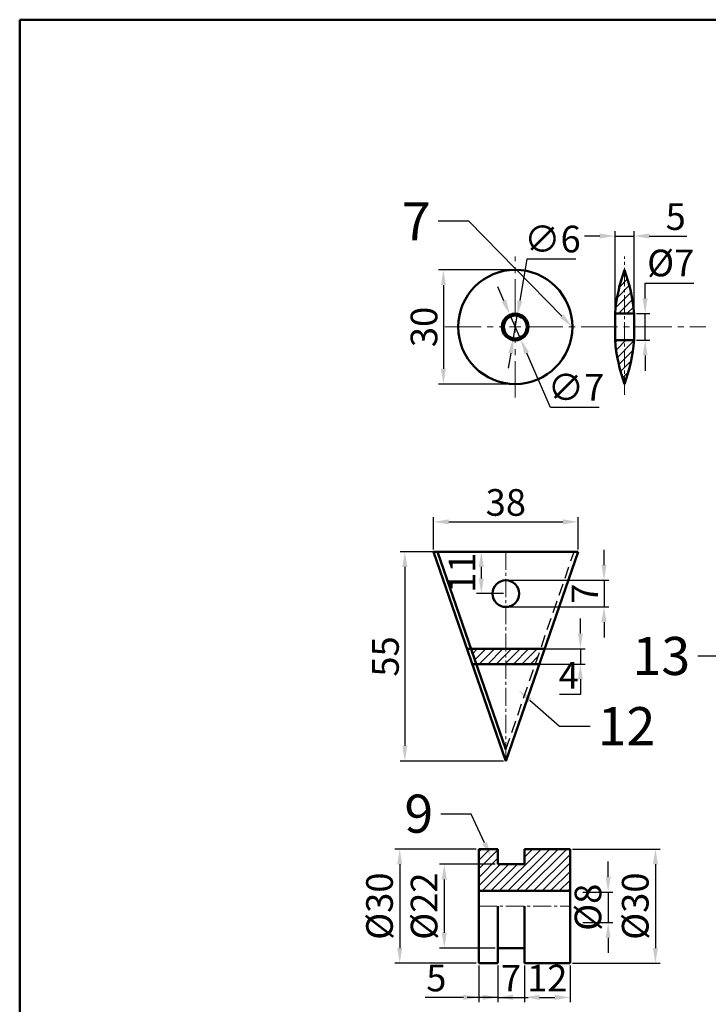
# Model space of a CAD drawing. Units: millimetres. Extents: x 376 to 1043, y -28 to 427.
# Tile 2 of 5: x 376 to 557, y 168 to 427. Entities that reach past the tile are written whole.
import ezdxf
from ezdxf import colors
from ezdxf.entities.mleader import LeaderData, LeaderLine
from ezdxf.math import Vec2, Vec3

# ---------------------------------------------------------------- set-up
doc = ezdxf.new("R2010")
doc.units = ezdxf.units.MM
doc.header["$LTSCALE"] = 0.5
doc.linetypes.add('CENTER2', pattern=[28.575, 19.05, -3.175, 3.175, -3.175])
doc.linetypes.add('DASHED', pattern=[19.05, 12.7, -6.35])
for name, color, linetype, lineweight in [('M-CNTR', 1, 'CENTER2', 18), ('M-DIMS', 2, 'Continuous', 25), ('M-HATC', 8, 'Continuous', 18), ('M-HIDN', 4, 'DASHED', 25), ('M-OUTL', 7, 'Continuous', 50)]:
    doc.layers.add(name, color=color, linetype=linetype, lineweight=lineweight)
doc.styles.get("Standard").update_dxf_attribs({"font": 'arial.ttf'})
doc.dimstyles.new('ISO-25', dxfattribs={"dimtxt": 7, "dimasz": 4, "dimexe": 1.25, "dimexo": 0.625, "dimtad": 1, "dimtoh": 1, "dimtxsty": 'Standard', "dimcen": 2.5, "dimadec": 0, "dimazin": 0, "dimtfac": 1, "dimtmove": 0, "dimatfit": 3, "dimfxl": 1, "dimarcsym": 0})

# ---------------------------------------------------------------- blocks, each defined once
blk = doc.blocks.new('*U36')
at = {"layer": 'M-CNTR', "color": 0, "transparency": 16777216}
for p, q in [((0, 3), (0, 18.5)), ((-18.5, 0), (-3, 0)), ((3, 0), (50.08, 0)), ((0, -18.5), (0, -3))]:
    blk.add_line(p, q, dxfattribs=at)
at = {"layer": 'M-CNTR', "color": 0, "linetype": 'Continuous', "transparency": 16777216}
for p, q in [((-1.5, 0), (1.5, 0)), ((0, -1.5), (0, 1.5))]:
    blk.add_line(p, q, dxfattribs=at)
blk = doc.blocks.new('*D37')
at = {"layer": 'Defpoints', "color": 0, "ltscale": 0.5, "transparency": 16777216}
for p in [(537.84, 370.17), (532.84, 346.29), (537.84, 346.29)]:
    blk.add_point(p, dxfattribs=at)
at = {"layer": 'M-DIMS', "color": 0, "lineweight": -2, "ltscale": 0.5, "transparency": 16777216}
for p, q in [((528.84, 370.17), (524.84, 370.17)), ((532.84, 346.91), (532.84, 371.42)), ((532.84, 370.17), (537.84, 370.17)), ((537.84, 346.91), (537.84, 371.42)), ((541.84, 370.17), (551.73, 370.17))]:
    blk.add_line(p, q, dxfattribs=at)
at = {"layer": 'M-DIMS', "color": 0, "ltscale": 0.5, "transparency": 16777216}
for points in [[(528.84, 370.84), (528.84, 369.5), (532.84, 370.17)], [(541.84, 370.84), (541.84, 369.5), (537.84, 370.17)]]:
    blk.add_solid(points, dxfattribs=at)
at = {"layer": 'M-DIMS', "color": 0, "ltscale": 0.5, "transparency": 16777216, "insert": (548.78, 374.36), "char_height": 7, "attachment_point": 5}
blk.add_mtext('5', dxfattribs=at)
blk = doc.blocks.new('*D38')
at = {"layer": 'Defpoints', "color": 0, "ltscale": 0.5, "transparency": 16777216}
for p in [(537.84, 349.79), (537.84, 342.79), (540.75, 342.79)]:
    blk.add_point(p, dxfattribs=at)
at = {"layer": 'M-DIMS', "color": 0, "lineweight": -2, "ltscale": 0.5, "transparency": 16777216}
for p, q in [((540.75, 353.79), (540.75, 357.79)), ((540.75, 357.79), (553.58, 357.79)), ((538.46, 349.79), (542, 349.79)), ((540.75, 342.79), (540.75, 349.79)), ((538.46, 342.79), (542, 342.79)), ((540.75, 338.79), (540.75, 334.79))]:
    blk.add_line(p, q, dxfattribs=at)
at = {"layer": 'M-DIMS', "color": 0, "ltscale": 0.5, "transparency": 16777216}
for points in [[(540.08, 353.79), (541.41, 353.79), (540.75, 349.79)], [(540.08, 338.79), (541.41, 338.79), (540.75, 342.79)]]:
    blk.add_solid(points, dxfattribs=at)
at = {"layer": 'M-DIMS', "color": 0, "ltscale": 0.5, "transparency": 16777216, "insert": (547.47, 362.18), "char_height": 7, "attachment_point": 5}
blk.add_mtext('%%C7', dxfattribs=at)
blk = doc.blocks.new('*D39')
at = {"layer": 'Defpoints', "color": 0, "ltscale": 0.5, "transparency": 16777216}
for p in [(506.64, 361.29), (487.76, 331.29), (506.64, 331.29)]:
    blk.add_point(p, dxfattribs=at)
at = {"layer": 'M-DIMS', "color": 0, "lineweight": -2, "ltscale": 0.5, "transparency": 16777216}
for p, q in [((506.01, 361.29), (486.51, 361.29)), ((487.76, 357.29), (487.76, 335.29)), ((506.01, 331.29), (486.51, 331.29))]:
    blk.add_line(p, q, dxfattribs=at)
at = {"layer": 'M-DIMS', "color": 0, "ltscale": 0.5, "transparency": 16777216}
for points in [[(487.09, 357.29), (488.42, 357.29), (487.76, 361.29)], [(487.09, 335.29), (488.42, 335.29), (487.76, 331.29)]]:
    blk.add_solid(points, dxfattribs=at)
at = {"layer": 'M-DIMS', "color": 0, "ltscale": 0.5, "transparency": 16777216, "insert": (483.56, 346.29), "char_height": 7, "attachment_point": 5, "rotation": 90}
blk.add_mtext('30', dxfattribs=at)
blk = doc.blocks.new('*D40')
at = {"layer": 'Defpoints', "color": 0, "ltscale": 0.5, "transparency": 16777216}
for p in [(505.24, 349.5), (508.04, 343.08)]:
    blk.add_point(p, dxfattribs=at)
at = {"layer": 'M-DIMS', "color": 0, "lineweight": -2, "ltscale": 0.5, "transparency": 16777216}
for p, q in [((503.64, 353.16), (502.04, 356.83)), ((505.24, 349.5), (508.04, 343.08)), ((515.86, 325.14), (509.64, 339.41)), ((528.69, 325.14), (515.86, 325.14))]:
    blk.add_line(p, q, dxfattribs=at)
at = {"layer": 'M-DIMS', "color": 0, "ltscale": 0.5, "transparency": 16777216}
for points in [[(504.25, 353.43), (503.03, 352.9), (505.24, 349.5)], [(510.25, 339.68), (509.03, 339.15), (508.04, 343.08)]]:
    blk.add_solid(points, dxfattribs=at)
at = {"layer": 'M-DIMS', "color": 0, "ltscale": 0.5, "transparency": 16777216, "insert": (522.59, 329.53), "char_height": 7, "attachment_point": 5}
blk.add_mtext('∅7', dxfattribs=at)
blk = doc.blocks.new('*D41')
at = {"layer": 'Defpoints', "color": 0, "ltscale": 0.5, "transparency": 16777216}
for p in [(507.15, 349.24), (506.13, 343.33)]:
    blk.add_point(p, dxfattribs=at)
at = {"layer": 'M-DIMS', "color": 0, "lineweight": -2, "ltscale": 0.5, "transparency": 16777216}
for p, q in [((509.68, 364.07), (507.82, 353.19)), ((522.51, 364.07), (509.68, 364.07)), ((506.13, 343.33), (507.15, 349.24)), ((505.46, 339.39), (504.78, 335.44))]:
    blk.add_line(p, q, dxfattribs=at)
at = {"layer": 'M-DIMS', "color": 0, "ltscale": 0.5, "transparency": 16777216}
for points in [[(507.16, 353.3), (508.48, 353.07), (507.15, 349.24)], [(504.8, 339.5), (506.12, 339.27), (506.13, 343.33)]]:
    blk.add_solid(points, dxfattribs=at)
at = {"layer": 'M-DIMS', "color": 0, "ltscale": 0.5, "transparency": 16777216, "insert": (516.41, 368.47), "char_height": 7, "attachment_point": 5}
blk.add_mtext('∅6', dxfattribs=at)
blk = doc.blocks.new('*D42')
at = {"layer": 'Defpoints', "color": 0, "ltscale": 0.5, "transparency": 16777216}
for p in [(502.03, 205.16), (487.99, 183.16), (502.03, 183.16)]:
    blk.add_point(p, dxfattribs=at)
at = {"layer": 'M-DIMS', "color": 0, "lineweight": -2, "ltscale": 0.5, "transparency": 16777216}
for p, q in [((501.4, 205.16), (486.74, 205.16)), ((487.99, 201.16), (487.99, 187.16)), ((501.4, 183.16), (486.74, 183.16))]:
    blk.add_line(p, q, dxfattribs=at)
at = {"layer": 'M-DIMS', "color": 0, "ltscale": 0.5, "transparency": 16777216}
for points in [[(487.32, 201.16), (488.65, 201.16), (487.99, 205.16)], [(487.32, 187.16), (488.65, 187.16), (487.99, 183.16)]]:
    blk.add_solid(points, dxfattribs=at)
at = {"layer": 'M-DIMS', "color": 0, "ltscale": 0.5, "transparency": 16777216, "insert": (483.59, 194.16), "char_height": 7, "attachment_point": 5, "rotation": 90}
blk.add_mtext('%%C22', dxfattribs=at)
blk = doc.blocks.new('*D43')
at = {"layer": 'Defpoints', "color": 0, "ltscale": 0.5, "transparency": 16777216}
for p in [(497.03, 209.16), (476.28, 179.16), (497.03, 179.16)]:
    blk.add_point(p, dxfattribs=at)
at = {"layer": 'M-DIMS', "color": 0, "lineweight": -2, "ltscale": 0.5, "transparency": 16777216}
for p, q in [((496.4, 209.16), (475.03, 209.16)), ((476.28, 205.16), (476.28, 183.16)), ((496.4, 179.16), (475.03, 179.16))]:
    blk.add_line(p, q, dxfattribs=at)
at = {"layer": 'M-DIMS', "color": 0, "ltscale": 0.5, "transparency": 16777216}
for points in [[(475.61, 205.16), (476.95, 205.16), (476.28, 209.16)], [(475.61, 183.16), (476.95, 183.16), (476.28, 179.16)]]:
    blk.add_solid(points, dxfattribs=at)
at = {"layer": 'M-DIMS', "color": 0, "ltscale": 0.5, "transparency": 16777216, "insert": (471.88, 194.16), "char_height": 7, "attachment_point": 5, "rotation": 90}
blk.add_mtext('%%C30', dxfattribs=at)
blk = doc.blocks.new('*D44')
at = {"layer": 'Defpoints', "color": 0, "ltscale": 0.5, "transparency": 16777216}
for p in [(497.03, 179.16), (502.03, 179.16), (502.03, 170.21)]:
    blk.add_point(p, dxfattribs=at)
at = {"layer": 'M-DIMS', "color": 0, "lineweight": -2, "ltscale": 0.5, "transparency": 16777216}
for p, q in [((497.03, 178.54), (497.03, 168.96)), ((502.03, 178.54), (502.03, 168.96)), ((493.03, 170.21), (482.96, 170.21)), ((502.03, 170.21), (497.03, 170.21)), ((506.03, 170.21), (510.03, 170.21))]:
    blk.add_line(p, q, dxfattribs=at)
at = {"layer": 'M-DIMS', "color": 0, "ltscale": 0.5, "transparency": 16777216}
for points in [[(493.03, 170.88), (493.03, 169.54), (497.03, 170.21)], [(506.03, 170.88), (506.03, 169.54), (502.03, 170.21)]]:
    blk.add_solid(points, dxfattribs=at)
at = {"layer": 'M-DIMS', "color": 0, "ltscale": 0.5, "transparency": 16777216, "insert": (485.9, 174.39), "char_height": 7, "attachment_point": 5}
blk.add_mtext('5', dxfattribs=at)
blk = doc.blocks.new('*D45')
at = {"layer": 'Defpoints', "color": 0, "ltscale": 0.5, "transparency": 16777216}
for p in [(502.03, 179.16), (509.03, 179.16), (509.03, 170.21)]:
    blk.add_point(p, dxfattribs=at)
at = {"layer": 'M-DIMS', "color": 0, "lineweight": -2, "ltscale": 0.5, "transparency": 16777216}
for p, q in [((502.03, 178.54), (502.03, 168.96)), ((509.03, 178.54), (509.03, 168.96)), ((498.03, 170.21), (494.03, 170.21)), ((502.03, 170.21), (509.03, 170.21)), ((513.03, 170.21), (517.03, 170.21))]:
    blk.add_line(p, q, dxfattribs=at)
at = {"layer": 'M-DIMS', "color": 0, "ltscale": 0.5, "transparency": 16777216}
for points in [[(498.03, 170.88), (498.03, 169.54), (502.03, 170.21)], [(513.03, 170.88), (513.03, 169.54), (509.03, 170.21)]]:
    blk.add_solid(points, dxfattribs=at)
at = {"layer": 'M-DIMS', "color": 0, "ltscale": 0.5, "transparency": 16777216, "insert": (505.53, 174.34), "char_height": 7, "attachment_point": 5}
blk.add_mtext('7', dxfattribs=at)
blk = doc.blocks.new('*D46')
at = {"layer": 'Defpoints', "color": 0, "ltscale": 0.5, "transparency": 16777216}
for p in [(509.03, 179.16), (521.03, 179.16), (521.03, 170.21)]:
    blk.add_point(p, dxfattribs=at)
at = {"layer": 'M-DIMS', "color": 0, "lineweight": -2, "ltscale": 0.5, "transparency": 16777216}
for p, q in [((509.03, 178.54), (509.03, 168.96)), ((521.03, 178.54), (521.03, 168.96)), ((513.03, 170.21), (517.03, 170.21))]:
    blk.add_line(p, q, dxfattribs=at)
at = {"layer": 'M-DIMS', "color": 0, "ltscale": 0.5, "transparency": 16777216}
for points in [[(513.03, 170.88), (513.03, 169.54), (509.03, 170.21)], [(517.03, 170.88), (517.03, 169.54), (521.03, 170.21)]]:
    blk.add_solid(points, dxfattribs=at)
at = {"layer": 'M-DIMS', "color": 0, "ltscale": 0.5, "transparency": 16777216, "insert": (515.03, 174.35), "char_height": 7, "attachment_point": 5}
blk.add_mtext('12', dxfattribs=at)
blk = doc.blocks.new('*D47')
at = {"layer": 'Defpoints', "color": 0, "ltscale": 0.5, "transparency": 16777216}
for p in [(523.77, 197.87), (523.77, 189.87), (531.04, 189.87)]:
    blk.add_point(p, dxfattribs=at)
at = {"layer": 'M-DIMS', "color": 0, "lineweight": -2, "ltscale": 0.5, "transparency": 16777216}
for p, q in [((531.04, 201.87), (531.04, 205.87)), ((524.4, 197.87), (532.29, 197.87)), ((531.04, 197.87), (531.04, 189.87)), ((524.4, 189.87), (532.29, 189.87)), ((531.04, 185.87), (531.04, 181.87))]:
    blk.add_line(p, q, dxfattribs=at)
at = {"layer": 'M-DIMS', "color": 0, "ltscale": 0.5, "transparency": 16777216}
for points in [[(530.37, 201.87), (531.7, 201.87), (531.04, 197.87)], [(530.37, 185.87), (531.7, 185.87), (531.04, 189.87)]]:
    blk.add_solid(points, dxfattribs=at)
at = {"layer": 'M-DIMS', "color": 0, "ltscale": 0.5, "transparency": 16777216, "insert": (526.64, 193.87), "char_height": 7, "attachment_point": 5, "rotation": 90}
blk.add_mtext('%%C8', dxfattribs=at)
blk = doc.blocks.new('*D48')
at = {"layer": 'Defpoints', "color": 0, "ltscale": 0.5, "transparency": 16777216}
for p in [(521.03, 209.16), (521.03, 179.16), (543.45, 179.16)]:
    blk.add_point(p, dxfattribs=at)
at = {"layer": 'M-DIMS', "color": 0, "lineweight": -2, "ltscale": 0.5, "transparency": 16777216}
for p, q in [((521.65, 209.16), (544.7, 209.16)), ((543.45, 205.16), (543.45, 183.16)), ((521.65, 179.16), (544.7, 179.16))]:
    blk.add_line(p, q, dxfattribs=at)
at = {"layer": 'M-DIMS', "color": 0, "ltscale": 0.5, "transparency": 16777216}
for points in [[(542.79, 205.16), (544.12, 205.16), (543.45, 209.16)], [(542.79, 183.16), (544.12, 183.16), (543.45, 179.16)]]:
    blk.add_solid(points, dxfattribs=at)
at = {"layer": 'M-DIMS', "color": 0, "ltscale": 0.5, "transparency": 16777216, "insert": (539.06, 194.16), "char_height": 7, "attachment_point": 5, "rotation": 90}
blk.add_mtext('%%C30', dxfattribs=at)
blk = doc.blocks.new('*D49')
at = {"layer": 'Defpoints', "color": 0, "ltscale": 0.5, "transparency": 16777216}
for p in [(523.16, 295.09), (485.16, 287.24), (523.16, 287.24)]:
    blk.add_point(p, dxfattribs=at)
at = {"layer": 'M-DIMS', "color": 0, "lineweight": -2, "ltscale": 0.5, "transparency": 16777216}
for p, q in [((485.16, 287.86), (485.16, 296.34)), ((489.16, 295.09), (519.16, 295.09)), ((523.16, 287.86), (523.16, 296.34))]:
    blk.add_line(p, q, dxfattribs=at)
at = {"layer": 'M-DIMS', "color": 0, "ltscale": 0.5, "transparency": 16777216}
for points in [[(489.16, 295.76), (489.16, 294.43), (485.16, 295.09)], [(519.16, 295.76), (519.16, 294.43), (523.16, 295.09)]]:
    blk.add_solid(points, dxfattribs=at)
at = {"layer": 'M-DIMS', "color": 0, "ltscale": 0.5, "transparency": 16777216, "insert": (504.16, 299.29), "char_height": 7, "attachment_point": 5}
blk.add_mtext('38', dxfattribs=at)
blk = doc.blocks.new('*D50')
at = {"layer": 'Defpoints', "color": 0, "ltscale": 0.5, "transparency": 16777216}
for p in [(504.16, 287.24), (497.72, 276.24), (504.16, 276.24)]:
    blk.add_point(p, dxfattribs=at)
at = {"layer": 'M-DIMS', "color": 0, "lineweight": -2, "ltscale": 0.5, "transparency": 16777216}
for p, q in [((503.53, 287.24), (496.47, 287.24)), ((497.72, 283.24), (497.72, 280.24)), ((503.53, 276.24), (496.47, 276.24))]:
    blk.add_line(p, q, dxfattribs=at)
at = {"layer": 'M-DIMS', "color": 0, "ltscale": 0.5, "transparency": 16777216}
for points in [[(497.05, 283.24), (498.38, 283.24), (497.72, 287.24)], [(497.05, 280.24), (498.38, 280.24), (497.72, 276.24)]]:
    blk.add_solid(points, dxfattribs=at)
at = {"layer": 'M-DIMS', "color": 0, "ltscale": 0.5, "transparency": 16777216, "insert": (493.58, 281.74), "char_height": 7, "attachment_point": 5, "rotation": 90}
blk.add_mtext('11', dxfattribs=at)
blk = doc.blocks.new('*D51')
at = {"layer": 'Defpoints', "color": 0, "ltscale": 0.5, "transparency": 16777216}
for p in [(504.16, 279.74), (504.16, 272.74), (529.95, 272.74)]:
    blk.add_point(p, dxfattribs=at)
at = {"layer": 'M-DIMS', "color": 0, "lineweight": -2, "ltscale": 0.5, "transparency": 16777216}
for p, q in [((529.95, 283.74), (529.95, 287.74)), ((504.78, 279.74), (531.2, 279.74)), ((529.95, 279.74), (529.95, 272.74)), ((504.78, 272.74), (531.2, 272.74)), ((529.95, 268.74), (529.95, 264.74))]:
    blk.add_line(p, q, dxfattribs=at)
at = {"layer": 'M-DIMS', "color": 0, "ltscale": 0.5, "transparency": 16777216}
for points in [[(529.28, 283.74), (530.61, 283.74), (529.95, 279.74)], [(529.28, 268.74), (530.61, 268.74), (529.95, 272.74)]]:
    blk.add_solid(points, dxfattribs=at)
at = {"layer": 'M-DIMS', "color": 0, "ltscale": 0.5, "transparency": 16777216, "insert": (525.82, 276.24), "char_height": 7, "attachment_point": 5, "rotation": 90}
blk.add_mtext('7', dxfattribs=at)
blk = doc.blocks.new('*D52')
at = {"layer": 'Defpoints', "color": 0, "ltscale": 0.5, "transparency": 16777216}
for p in [(511.98, 261.74), (511.91, 257.74), (523.75, 257.74)]:
    blk.add_point(p, dxfattribs=at)
at = {"layer": 'M-DIMS', "color": 0, "lineweight": -2, "ltscale": 0.5, "transparency": 16777216}
for p, q in [((523.75, 265.74), (523.75, 269.74)), ((512.61, 261.74), (525, 261.74)), ((523.75, 261.74), (523.75, 257.74)), ((512.54, 257.74), (525, 257.74)), ((523.75, 253.74), (523.75, 249.74)), ((523.75, 249.74), (518.28, 249.74))]:
    blk.add_line(p, q, dxfattribs=at)
at = {"layer": 'M-DIMS', "color": 0, "ltscale": 0.5, "transparency": 16777216}
for points in [[(523.08, 265.74), (524.42, 265.74), (523.75, 261.74)], [(523.08, 253.74), (524.42, 253.74), (523.75, 257.74)]]:
    blk.add_solid(points, dxfattribs=at)
at = {"layer": 'M-DIMS', "color": 0, "ltscale": 0.5, "transparency": 16777216, "insert": (520.71, 253.86), "char_height": 7, "attachment_point": 5}
blk.add_mtext('4', dxfattribs=at)
blk = doc.blocks.new('*D53')
at = {"layer": 'Defpoints', "color": 0, "ltscale": 0.5, "transparency": 16777216}
for p in [(504.16, 287.24), (477.63, 232.24), (504.16, 232.24)]:
    blk.add_point(p, dxfattribs=at)
at = {"layer": 'M-DIMS', "color": 0, "lineweight": -2, "ltscale": 0.5, "transparency": 16777216}
for p, q in [((503.53, 287.24), (476.38, 287.24)), ((477.63, 283.24), (477.63, 236.24)), ((503.53, 232.24), (476.38, 232.24))]:
    blk.add_line(p, q, dxfattribs=at)
at = {"layer": 'M-DIMS', "color": 0, "ltscale": 0.5, "transparency": 16777216}
for points in [[(476.96, 283.24), (478.29, 283.24), (477.63, 287.24)], [(476.96, 236.24), (478.29, 236.24), (477.63, 232.24)]]:
    blk.add_solid(points, dxfattribs=at)
at = {"layer": 'M-DIMS', "color": 0, "ltscale": 0.5, "transparency": 16777216, "insert": (473.44, 259.74), "char_height": 7, "attachment_point": 5, "rotation": 90}
blk.add_mtext('55', dxfattribs=at)

msp = doc.modelspace()

# ---------------------------------------------------------------- hatches: boundary and pattern name
at = {"layer": 'M-HATC', "ltscale": 0.5}
h = msp.add_hatch(dxfattribs=at)
h.set_pattern_fill('ANSI31', color=256, scale=0.5)
h.set_pattern_definition([(45, (330.2008, 161.9684), (-1.122532, 1.122532), [])])
h.paths.add_polyline_path([(535.338, 361.287), (535.338, 349.787), (537.838, 349.787, 0.0643531)])
h.paths.add_polyline_path([(535.338, 361.287, 0.0643531), (532.838, 349.787), (535.338, 349.787)])
h.paths.add_polyline_path([(535.338, 342.787), (532.838, 342.787, 0.0643531), (535.338, 331.287)])
h.paths.add_polyline_path([(537.838, 342.787), (535.338, 342.787), (535.338, 331.287, 0.0643531)])
h = msp.add_hatch(dxfattribs=at)
h.set_pattern_fill('ANSI31', color=256, scale=0.5)
h.set_pattern_definition([(45, (121.9719, 95.8301), (-1.122532, 1.122532), [])])
h.paths.add_polyline_path([(504.16, 261.739), (495.027, 261.739), (496.409, 257.739), (504.16, 257.739)])
h.paths.add_polyline_path([(513.293, 261.739), (504.16, 261.739), (504.16, 257.739), (511.911, 257.739)])
h = msp.add_hatch(dxfattribs=at)
h.set_pattern_fill('ANSI31', color=256, scale=0.5)
h.set_pattern_definition([(45, (221.8312, 5.101), (-1.122532, 1.122532), [])])
h.paths.add_polyline_path([(509.03, 205.162), (502.03, 205.162), (502.03, 209.162), (497.03, 209.162), (497.03, 198.162), (521.03, 198.162), (521.03, 209.162), (509.03, 209.162)])

# ---------------------------------------------------------------- linework, layer by layer
at = {"layer": 'M-CNTR', "ltscale": 0.5}
for p, q in [((535.338, 328.457), (535.338, 364.808)), ((504.16, 287.239), (504.16, 232.239)), ((497.03, 194.162), (521.03, 194.162))]:
    msp.add_line(p, q, dxfattribs=at)
at = {"layer": 'M-HIDN', "ltscale": 0.5}
msp.add_line((504.16, 235.301), (522.102, 287.239), dxfattribs=at)
at = {"layer": 'M-OUTL', "ltscale": 0.5}
for p, q in [((532.838, 346.287), (532.838, 349.787)), ((532.838, 349.787), (537.838, 349.787)), ((537.838, 349.787), (537.838, 342.787)), ((532.838, 342.787), (532.838, 346.287)), ((537.838, 342.787), (532.838, 342.787)), ((485.16, 287.239), (523.16, 287.239)), ((504.16, 232.239), (485.16, 287.239)), ((504.16, 235.301), (486.218, 287.239)), ((504.16, 232.239), (523.16, 287.239)), ((514.351, 261.739), (493.969, 261.739)), ((512.969, 257.739), (495.351, 257.739)), ((497.03, 209.162), (497.03, 179.162)), ((502.03, 209.162), (497.03, 209.162)), ((502.03, 205.162), (502.03, 209.162)), ((521.03, 209.162), (509.03, 209.162)), ((509.03, 209.162), (509.03, 205.162)), ((521.03, 179.162), (521.03, 209.162)), ((509.03, 205.162), (502.03, 205.162)), ((497.03, 198.162), (521.03, 198.162)), ((502.03, 179.162), (502.03, 194.162)), ((509.03, 194.162), (509.03, 179.162)), ((502.03, 183.162), (509.03, 183.162)), ((497.03, 179.162), (502.03, 179.162)), ((509.03, 179.162), (521.03, 179.162))]:
    msp.add_line(p, q, dxfattribs=at)
msp.add_lwpolyline([(376.448, 426.986), (1042.916, 426.986), (1042.916, -28.377), (376.448, -28.377)], close=True, dxfattribs=at)
for centre, radius in [((506.639, 346.287), 15), ((506.639, 346.287), 3.5), ((506.639, 346.287), 3), ((504.16, 276.239), 3.5)]:
    msp.add_circle(centre, radius, dxfattribs=at)
for centre, start, end in [((578.578, 345.865), 160.37106, 175.09939), ((492.097, 345.865), 4.90061, 19.62894), ((578.578, 346.709), 184.90061, 199.62894), ((492.097, 346.709), 340.37106, 355.09939)]:
    msp.add_arc(centre, 45.908, start, end, dxfattribs=at)

# ---------------------------------------------------------------- block references
at = {"layer": 'M-CNTR'}
msp.add_blockref('*U36', (506.639, 346.287), dxfattribs=at)

# ---------------------------------------------------------------- dimensions: what is measured, and where the dimension line sits
at = {"layer": 'M-DIMS', "ltscale": 0.5}
for base, p1, p2, picture, middle in [((537.838, 370.17), (532.838, 346.287), (537.838, 346.287), '*D37', (548.783, 374.355)), ((523.16, 295.092), (485.16, 287.239), (523.16, 287.239), '*D49', (504.16, 299.293)), ((509.03, 170.21), (502.03, 179.162), (509.03, 179.162), '*D45', (505.53, 174.335)), ((521.03, 170.21), (509.03, 179.162), (521.03, 179.162), '*D46', (515.03, 174.35))]:
    dim = msp.add_linear_dim(base=base, p1=p1, p2=p2, dimstyle='ISO-25', override={"dimclrd": 0, "dimclre": 0, "dimclrt": 0}, dxfattribs=at)
    dim.commit()
    dim.dimension.update_dxf_attribs({"geometry": picture, "text_midpoint": middle})
for p1, p2, picture, middle in [((506.133, 343.33), (507.145, 349.244), '*D41', (516.408, 364.074)), ((505.241, 349.495), (508.038, 343.078), '*D40', (522.587, 325.138))]:
    dim = msp.add_diameter_dim_2p(p1=p1, p2=p2, dimstyle='ISO-25', override={"dimclrd": 0, "dimclre": 0, "dimclrt": 0}, dxfattribs=at)
    dim.commit()
    dim.dimension.update_dxf_attribs({"geometry": picture, "text_midpoint": middle, "dimtype": 163})
for base, p1, p2, picture, middle in [((540.746, 342.787), (537.838, 349.787), (537.838, 342.787), '*D38', (547.473, 357.787)), ((531.037, 189.868), (523.775, 197.868), (523.775, 189.868), '*D47', (531.037, 193.868))]:
    dim = msp.add_linear_dim(base=base, p1=p1, p2=p2, angle=90, text='%%C<>', dimstyle='ISO-25', override={"dimclrd": 0, "dimclre": 0, "dimclrt": 0}, dxfattribs=at)
    dim.commit()
    dim.dimension.update_dxf_attribs({"geometry": picture, "text_midpoint": middle, "dimtype": 160})
dim = msp.add_aligned_dim(p1=(506.639, 361.287), p2=(506.639, 331.287), distance=-18.882, dimstyle='ISO-25', override={"dimclrd": 0, "dimclre": 0, "dimclrt": 0}, dxfattribs=at)
dim.commit()
dim.dimension.update_dxf_attribs({"geometry": '*D39', "text_midpoint": (483.556, 346.287)})
for base, p1, p2, picture, middle in [((477.626, 232.239), (504.16, 287.239), (504.16, 232.239), '*D53', (473.442, 259.739)), ((497.716, 276.239), (504.16, 287.239), (504.16, 276.239), '*D50', (493.577, 281.739)), ((523.751, 257.739), (511.982, 261.739), (511.911, 257.739), '*D52', (520.705, 253.864))]:
    dim = msp.add_linear_dim(base=base, p1=p1, p2=p2, angle=90, dimstyle='ISO-25', override={"dimclrd": 0, "dimclre": 0, "dimclrt": 0}, dxfattribs=at)
    dim.commit()
    dim.dimension.update_dxf_attribs({"geometry": picture, "text_midpoint": middle})
dim = msp.add_linear_dim(base=(529.947, 272.739), p1=(504.16, 279.739), p2=(504.16, 272.739), angle=270, dimstyle='ISO-25', override={"dimclrd": 0, "dimclre": 0, "dimclrt": 0}, dxfattribs=at)
dim.commit()
dim.dimension.update_dxf_attribs({"geometry": '*D51', "text_midpoint": (529.947, 276.239), "dimtype": 161})
for base, p1, p2, picture, middle in [((476.279, 179.162), (497.03, 209.162), (497.03, 179.162), '*D43', (471.884, 194.162)), ((543.453, 179.162), (521.03, 209.162), (521.03, 179.162), '*D48', (539.058, 194.162)), ((487.985, 183.162), (502.03, 205.162), (502.03, 183.162), '*D42', (483.591, 194.162))]:
    dim = msp.add_linear_dim(base=base, p1=p1, p2=p2, angle=90, text='%%C<>', dimstyle='ISO-25', override={"dimclrd": 0, "dimclre": 0, "dimclrt": 0}, dxfattribs=at)
    dim.commit()
    dim.dimension.update_dxf_attribs({"geometry": picture, "text_midpoint": middle})
dim = msp.add_linear_dim(base=(502.03, 170.21), p1=(497.03, 179.162), p2=(502.03, 179.162), dimstyle='ISO-25', override={"dimclrd": 0, "dimclre": 0, "dimclrt": 0}, dxfattribs=at)
dim.commit()
dim.dimension.update_dxf_attribs({"geometry": '*D44', "text_midpoint": (485.901, 170.21), "dimtype": 160})

# ---------------------------------------------------------------- leaders
ml = msp.add_multileader_mtext('Standard', dxfattribs=at)
ml.set_content('7', color=256)
ml.set_leader_properties()
ml.build(insert=Vec2(0, 0))
ctx = ml.context
ctx.base_point, ctx.char_height, ctx.plane_origin = Vec3(475.941, 374.029), 10, Vec3(502.542, 359.952)
ctx.text_align_type = 2
notes = []
notes.append((ctx, [(0, (1, 1, 0), (494.414, 374.029), (-1, 0), 8, [(0, [(521.639, 346.287)], 0, [])])]))
ctx.mtext.insert, ctx.mtext.alignment, ctx.mtext.flow_direction = Vec3(484.414, 379.029), 3, 5
ml = msp.add_multileader_mtext('Standard', dxfattribs=at)
ml.set_content('13', color=256)
ml.set_leader_properties()
ml.build(insert=Vec2(0, 0))
ctx = ml.context
ctx.base_point, ctx.char_height, ctx.plane_origin = Vec3(537.2, 259.791), 10, Vec3(584.958, 241.419)
ctx.text_align_type = 2
notes.append((ctx, [(0, (1, 1, 0), (562.584, 259.791), (-1, 0), 8, [(0, [(584.958, 241.419)], 0, [])])]))
ctx.mtext.insert, ctx.mtext.alignment, ctx.mtext.flow_direction = Vec3(552.584, 264.879), 3, 5
ml = msp.add_multileader_mtext('Standard', dxfattribs=at)
ml.set_content('12', color=256)
ml.set_leader_properties()
ml.build(insert=Vec2(0, 0))
ctx = ml.context
ctx.base_point, ctx.char_height, ctx.plane_origin = Vec3(526.294, 241.441), 10, Vec3(507.467, 250.871)
notes.append((ctx, [(0, (1, 1, 0), (518.294, 241.441), (1, 0), 8, [(0, [(507.467, 250.871)], 0, [])])]))
ctx.mtext.insert, ctx.mtext.flow_direction = Vec3(528.294, 246.441), 5
ml = msp.add_multileader_mtext('Standard', dxfattribs=at)
ml.set_content('9', color=256)
ml.set_leader_properties()
ml.build(insert=Vec2(0, 0))
ctx = ml.context
ctx.base_point, ctx.char_height, ctx.plane_origin = Vec3(476.508, 218.364), 10, Vec3(500.265, 207.131)
ctx.text_align_type = 2
notes.append((ctx, [(0, (1, 1, 0), (495.083, 218.364), (-1, 0), 8, [(0, [(500.265, 207.131)], 0, [])])]))
ctx.mtext.insert, ctx.mtext.alignment, ctx.mtext.flow_direction = Vec3(485.083, 223.449), 3, 5
for ctx, leaders in notes:
    for number, flags, end, landing, length, lines in leaders:
        leader = LeaderData()
        leader.index, (leader.has_last_leader_line, leader.has_dogleg_vector, leader.attachment_direction) = number, flags
        leader.last_leader_point, leader.dogleg_vector, leader.dogleg_length = Vec3(end), Vec3(landing), length
        for number, points, colour, breaks in lines:
            line = LeaderLine()
            line.index, line.vertices, line.color, line.breaks = number, Vec3.list(points), colors.encode_raw_color(colour), breaks
            leader.lines.append(line)
        ctx.leaders.append(leader)

doc.saveas('drawing.dxf')
